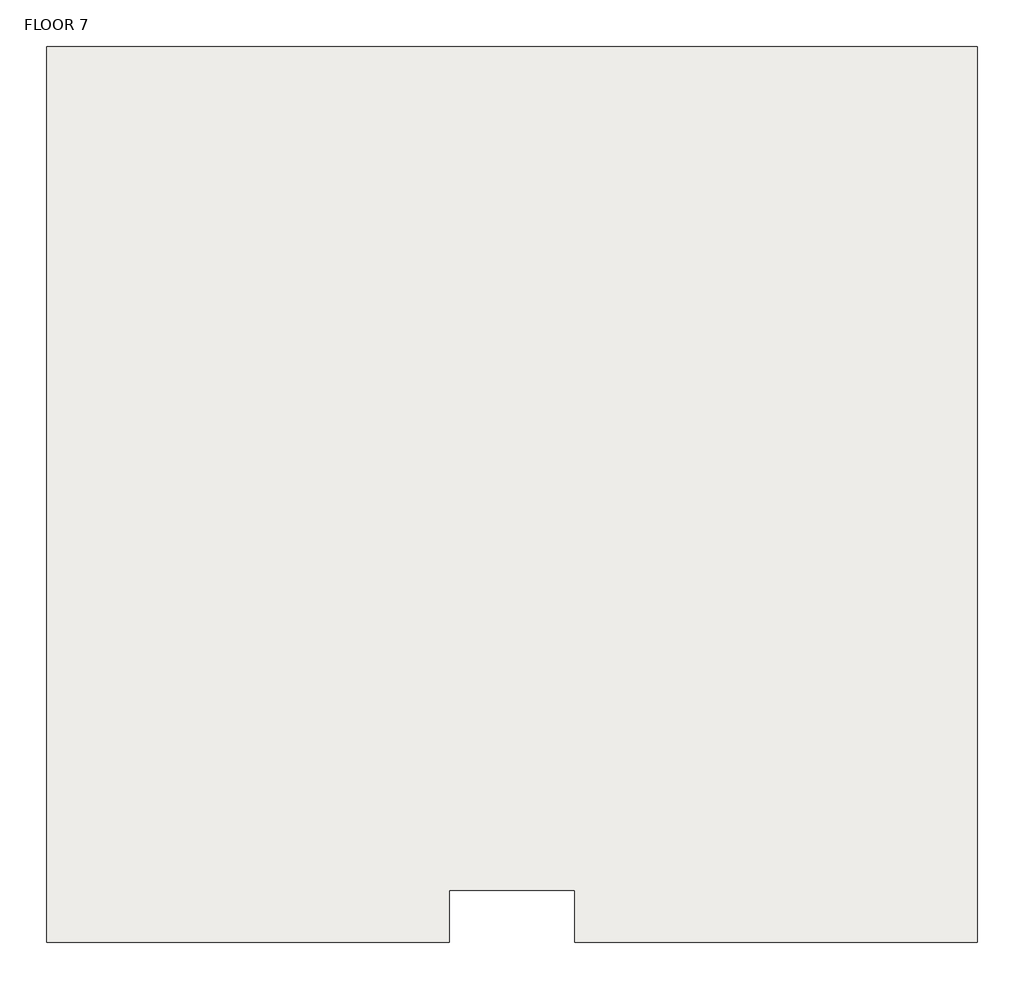
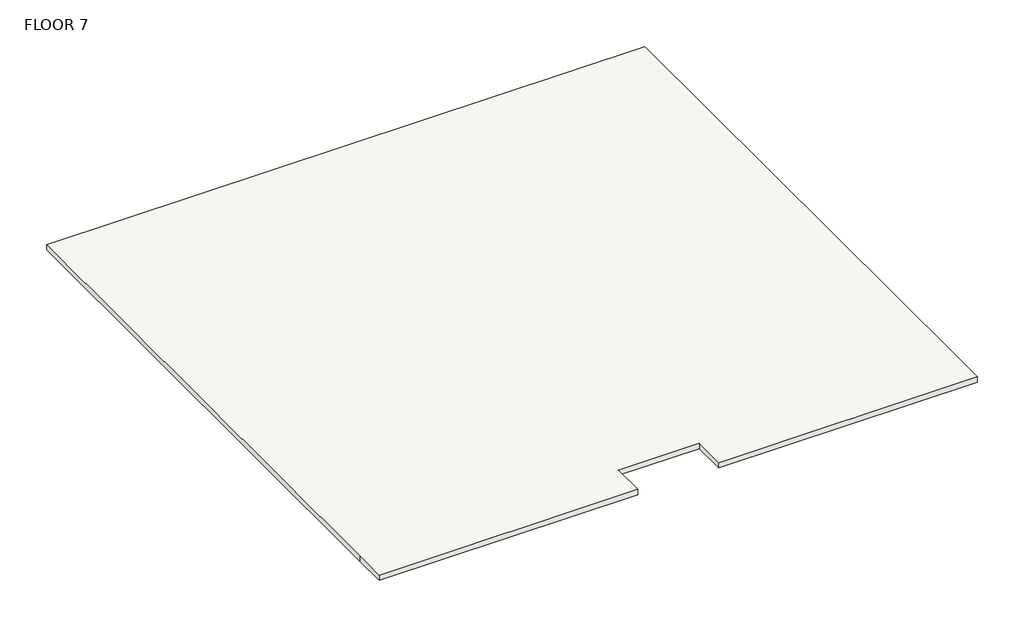
# One storey, incomplete: 1 roof.
"""IFC4 building model written with IfcOpenShell, lengths in millimetres."""

from ifc_helpers import new_model, si_unit, frame, origin, place, context, project, spatial, polyline, outline, extrude, element, save

model = new_model("IFC4")

# Units and contexts
model_context = context("Model", 3, world=origin())
ifc_project = project(units=[si_unit("LENGTHUNIT", "METRE", prefix="MILLI")], contexts=[model_context])

# Site, building, storey
site = spatial("IfcSite", under=ifc_project)
building = spatial("IfcBuilding", under=site)
storey = spatial("IfcBuildingStorey", under=building, Name="FLOOR 7", Elevation=12592.3725604)

# Roof
placement = place(None, origin())
element("IfcRoof", 1, ObjectType="ROOFING 6\"", at=placement, inside=storey, context=model_context, shape_type="SweptSolid", body=[
    extrude(outline(polyline([(-3159.4137331, -7822.4593836), (-5369.2137331, -7822.4593836), (-5369.2137331, -8736.8593836), (-12430.4137331, -8736.8593836), (-12430.4137331, -7822.4593836), (-12430.4137331, 6987.3281164), (3901.7862669, 6987.3281164), (3901.7862669, -7822.4593836), (3901.7862669, -8736.8593836), (-3159.4137331, -8736.8593836), (-3159.4137331, -7822.4593836)])), frame((0.0, 0.0, 12592.3725604), z_axis=(0.0, 0.0, 1.0), x_axis=(1.0, 0.0, 0.0)), (0.0, 0.0, 1.0), 152.4),
])

save(model, "model.ifc")

# Revit data of these elements
# Type "ROOFING 6\""
#   Assembly Code = "B1020"
#   Layers, outside or top first: 0' - 6" no material (function 1)
# Element 1 (IfcRoof, "ROOFING 6\"")
#   built-in parameter 1001705 = 41.8136 (stored number, unit not read)
#   built-in parameter 1001710 = 33615
#   Phase Created = New Construction
#   Materials on its faces: "Default Roof", "Clad - White"
# Materials
#   "Default Roof": colour RGB 88 101 114, transparency 0, Cost = 0
#   "Clad - White": class "Wood", colour RGB 242 242 238, transparency 0, Cost = 0
